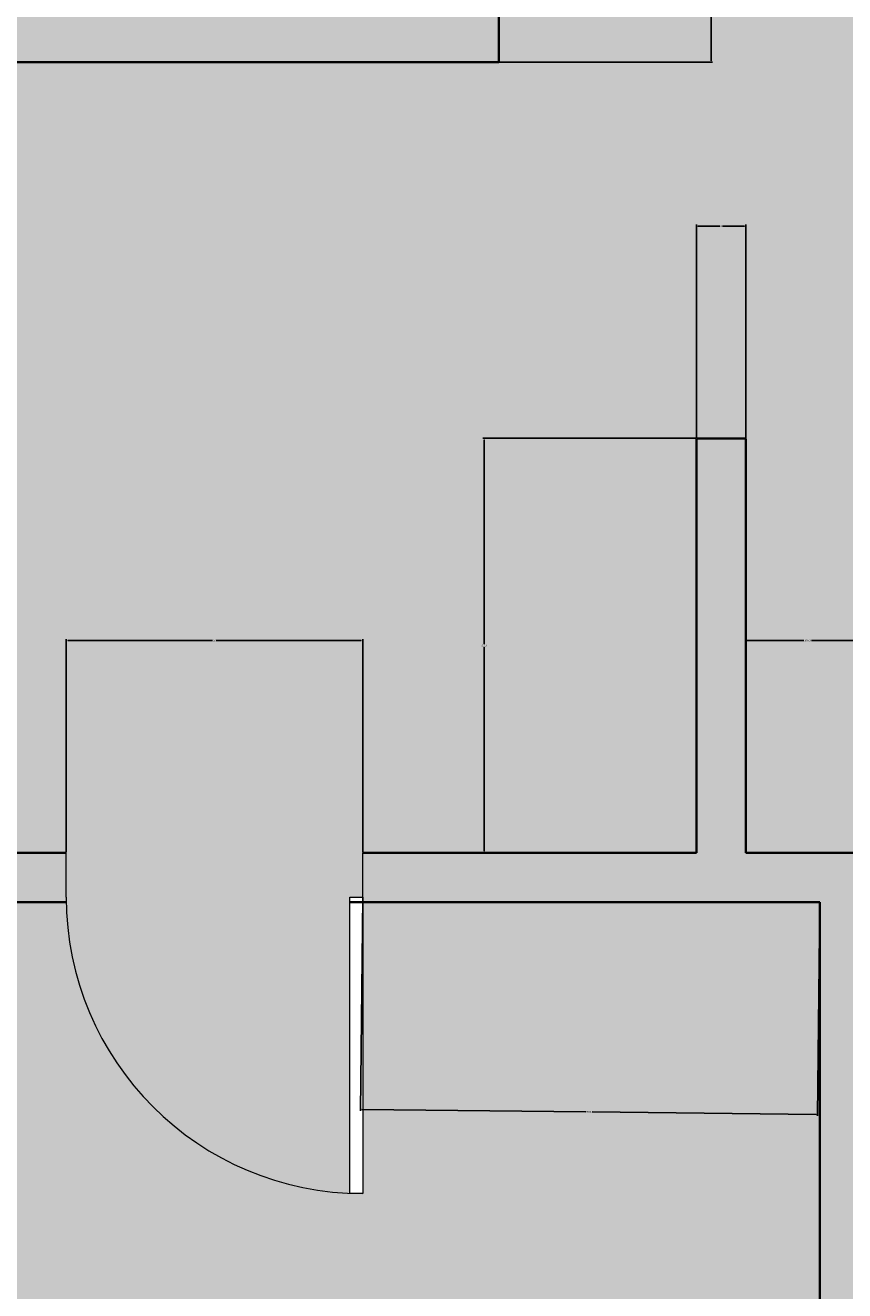
# Model space of a CAD drawing. Units: inches. Extents: x 3024 to 3952, y 1308 to 1863.
# Tile 3 of 29: x 3175 to 3275, y 1479 to 1633. Entities that reach past the tile are written whole.
import ezdxf

# ---------------------------------------------------------------- set-up
doc = ezdxf.new("R2010")
doc.units = ezdxf.units.IN
for name, color, linetype, lineweight in [('A-ANNO-DIMS', 2, 'Continuous', 18), ('A-DOOR', 4, 'Continuous', 18), ('A-FLOR-TILE-PATT', 7, 'Continuous', 13), ('A-WALL', 7, 'Continuous', 35)]:
    doc.layers.add(name, color=color, linetype=linetype, lineweight=lineweight)
doc.layers.add('A-FLOR-PATT', color=254, linetype='Continuous', lineweight=13, true_color=0xfeeab9)
doc.layers.add('A-WALL-PATT', color=254, linetype='Continuous', lineweight=13, true_color=0xcecce6)
doc.styles.get("Standard").update_dxf_attribs({"font": 'arial.ttf'})
doc.dimstyles.get("Standard").update_dxf_attribs({"dimtxt": 0.18, "dimasz": 0.18, "dimexe": 0.18, "dimexo": 0.0625, "dimgap": 0.09, "dimtad": 0, "dimtih": 1, "dimtoh": 1, "dimdec": 4, "dimzin": 0, "dimdsep": 46, "dimtxsty": 'Standard', "dimcen": 0.09, "dimadec": 0, "dimazin": 0, "dimtfac": 1, "dimtdec": 4, "dimtofl": 0, "dimtmove": 0, "dimatfit": 3, "dimfxl": 1, "dimtolj": 1, "dimtzin": 0, "dimarcsym": 0})

# ---------------------------------------------------------------- blocks, each defined once
blk = doc.blocks.new('*U2')
for p, q in [((0, 0), (0, -6)), ((40, 0), (40, -6))]:
    blk.add_line(p, q)
blk.add_lwpolyline([(0, 0), (0, 40), (1.75, 40), (1.75, 0)], close=True)
blk.add_arc((0, 0), 40, 0, 90)
blk = doc.blocks.new('*D52')
at = {"layer": 'A-ANNO-DIMS', "color": 0, "lineweight": -2, "transparency": 16777216}
for p, q in [((3180.24, 1532.67), (3180.24, 1558.56)), ((3216.24, 1532.67), (3216.24, 1558.56)), ((3180.42, 1558.38), (3198.02, 1558.38)), ((3216.06, 1558.38), (3198.46, 1558.38))]:
    blk.add_line(p, q, dxfattribs=at)
at = {"layer": 'A-ANNO-DIMS', "color": 0, "transparency": 16777216}
for points in [[(3180.42, 1558.41), (3180.42, 1558.35), (3180.24, 1558.38)], [(3216.06, 1558.41), (3216.06, 1558.35), (3216.24, 1558.38)]]:
    blk.add_solid(points, dxfattribs=at)
at = {"layer": 'Defpoints', "color": 0, "transparency": 16777216}
for p in [(3216.24, 1558.38), (3180.24, 1532.61), (3216.24, 1532.61)]:
    blk.add_point(p, dxfattribs=at)
at = {"layer": 'A-ANNO-DIMS', "color": 0, "transparency": 16777216, "insert": (3198.24, 1558.38), "char_height": 0.18, "attachment_point": 5}
blk.add_mtext('\\A1;36', dxfattribs=at)
blk = doc.blocks.new('*D55')
at = {"layer": 'A-ANNO-DIMS', "color": 0, "lineweight": -2, "transparency": 16777216}
for p, q in [((3216.24, 1527.14), (3215.96, 1501.25)), ((3271.76, 1526.54), (3271.48, 1500.65)), ((3216.14, 1501.43), (3243.33, 1501.14)), ((3271.31, 1500.83), (3244.12, 1501.13))]:
    blk.add_line(p, q, dxfattribs=at)
at = {"layer": 'A-ANNO-DIMS', "color": 0, "transparency": 16777216}
for points in [[(3216.14, 1501.46), (3216.14, 1501.4), (3215.96, 1501.43)], [(3271.31, 1500.86), (3271.31, 1500.8), (3271.49, 1500.83)]]:
    blk.add_solid(points, dxfattribs=at)
at = {"layer": 'Defpoints', "color": 0, "transparency": 16777216}
for p in [(3216.24, 1527.21), (3271.76, 1526.61), (3215.96, 1501.43)]:
    blk.add_point(p, dxfattribs=at)
at = {"layer": 'A-ANNO-DIMS', "color": 0, "transparency": 16777216, "insert": (3243.72, 1501.13), "char_height": 0.18, "attachment_point": 5}
blk.add_mtext('\\A1;55.53', dxfattribs=at)
blk = doc.blocks.new('*D59')
at = {"layer": 'A-ANNO-DIMS', "color": 0, "lineweight": -2, "transparency": 16777216}
for p, q in [((3232.83, 1649.9), (3258.72, 1649.9)), ((3258.54, 1649.72), (3258.54, 1639.43)), ((3258.54, 1628.79), (3258.54, 1639.07)), ((3232.83, 1628.61), (3258.72, 1628.61))]:
    blk.add_line(p, q, dxfattribs=at)
at = {"layer": 'A-ANNO-DIMS', "color": 0, "transparency": 16777216}
for points in [[(3258.51, 1649.72), (3258.57, 1649.72), (3258.54, 1649.9)], [(3258.51, 1628.79), (3258.57, 1628.79), (3258.54, 1628.61)]]:
    blk.add_solid(points, dxfattribs=at)
at = {"layer": 'Defpoints', "color": 0, "transparency": 16777216}
for p in [(3232.76, 1649.9), (3232.76, 1628.61), (3258.54, 1628.61)]:
    blk.add_point(p, dxfattribs=at)
at = {"layer": 'A-ANNO-DIMS', "color": 0, "transparency": 16777216, "insert": (3258.54, 1639.25), "char_height": 0.18, "attachment_point": 5}
blk.add_mtext('\\A1;21.29', dxfattribs=at)
blk = doc.blocks.new('*D64')
at = {"layer": 'A-ANNO-DIMS', "color": 0, "lineweight": -2, "transparency": 16777216}
for p, q in [((3256.7, 1582.94), (3230.81, 1582.94)), ((3230.99, 1582.76), (3230.99, 1557.95)), ((3230.99, 1532.79), (3230.99, 1557.59)), ((3256.7, 1532.61), (3230.81, 1532.61))]:
    blk.add_line(p, q, dxfattribs=at)
at = {"layer": 'A-ANNO-DIMS', "color": 0, "transparency": 16777216}
for points in [[(3230.96, 1582.76), (3231.02, 1582.76), (3230.99, 1582.94)], [(3230.96, 1532.79), (3231.02, 1532.79), (3230.99, 1532.61)]]:
    blk.add_solid(points, dxfattribs=at)
at = {"layer": 'Defpoints', "color": 0, "transparency": 16777216}
for p in [(3230.99, 1582.94), (3256.76, 1582.94), (3256.76, 1532.61)]:
    blk.add_point(p, dxfattribs=at)
at = {"layer": 'A-ANNO-DIMS', "color": 0, "transparency": 16777216, "insert": (3230.99, 1557.77), "char_height": 0.18, "attachment_point": 5}
blk.add_mtext('\\A1;50.33', dxfattribs=at)
blk = doc.blocks.new('*D65')
at = {"layer": 'A-ANNO-DIMS', "color": 0, "lineweight": -2, "transparency": 16777216}
for p, q in [((3262.76, 1532.67), (3262.76, 1558.56)), ((3277.76, 1532.67), (3277.76, 1558.56)), ((3262.94, 1558.38), (3269.81, 1558.38)), ((3277.58, 1558.38), (3270.72, 1558.38))]:
    blk.add_line(p, q, dxfattribs=at)
at = {"layer": 'A-ANNO-DIMS', "color": 0, "transparency": 16777216}
for points in [[(3262.94, 1558.41), (3262.94, 1558.35), (3262.76, 1558.38)], [(3277.58, 1558.41), (3277.58, 1558.35), (3277.76, 1558.38)]]:
    blk.add_solid(points, dxfattribs=at)
at = {"layer": 'Defpoints', "color": 0, "transparency": 16777216}
for p in [(3277.76, 1558.38), (3262.76, 1532.61), (3277.76, 1532.61)]:
    blk.add_point(p, dxfattribs=at)
at = {"layer": 'A-ANNO-DIMS', "color": 0, "transparency": 16777216, "insert": (3270.26, 1558.38), "char_height": 0.18, "attachment_point": 5}
blk.add_mtext('\\A1;15.003', dxfattribs=at)
blk = doc.blocks.new('*D66')
at = {"layer": 'A-ANNO-DIMS', "color": 0, "lineweight": -2, "transparency": 16777216}
for p, q in [((3256.76, 1583), (3256.76, 1608.89)), ((3256.94, 1608.71), (3259.61, 1608.71)), ((3262.58, 1608.71), (3259.91, 1608.71)), ((3262.76, 1583), (3262.76, 1608.89))]:
    blk.add_line(p, q, dxfattribs=at)
at = {"layer": 'A-ANNO-DIMS', "color": 0, "transparency": 16777216}
for points in [[(3256.94, 1608.74), (3256.94, 1608.68), (3256.76, 1608.71)], [(3262.58, 1608.74), (3262.58, 1608.68), (3262.76, 1608.71)]]:
    blk.add_solid(points, dxfattribs=at)
at = {"layer": 'Defpoints', "color": 0, "transparency": 16777216}
for p in [(3262.76, 1608.71), (3256.76, 1582.94), (3262.76, 1582.94)]:
    blk.add_point(p, dxfattribs=at)
at = {"layer": 'A-ANNO-DIMS', "color": 0, "transparency": 16777216, "insert": (3259.76, 1608.71), "char_height": 0.18, "attachment_point": 5}
blk.add_mtext('\\A1;6', dxfattribs=at)

msp = doc.modelspace()

# ---------------------------------------------------------------- hatches: boundary and pattern name
at = {"layer": 'A-FLOR-PATT', "transparency": 33554528}
h = msp.add_hatch(color=256, dxfattribs=at)
h.dxf.hatch_style = 1
h.paths.add_polyline_path([(3460.764, 1688.6064), (3412.764, 1688.6064), (3412.764, 1694.6064), (3460.764, 1694.6064), (3460.764, 1778.6064), (3406.764, 1778.6064), (3406.764, 1759.9514), (3318.2981, 1759.9514), (3318.2981, 1658.6064), (3322.5356, 1658.6064), (3322.5356, 1652.6064), (3292.764, 1652.6064), (3292.764, 1778.6064), (3106.764, 1778.6064), (3106.764, 1628.6064), (3172.764, 1628.6064), (3172.764, 1532.6064), (3166.764, 1532.6064), (3166.764, 1628.6064), (3106.764, 1628.6064), (3106.764, 1356.8452), (3202.812, 1356.8452), (3202.812, 1354.2534), (3202.812, 1353.8388), (3202.812, 1351.1212), (3202.812, 1347.8452), (3277.764, 1347.8452), (3277.764, 1353.8452), (3277.764, 1356.8452), (3277.764, 1442.6064), (3460.764, 1442.6064)])
h.paths.add_polyline_path([(3216.238, 1527.2064), (3216.238, 1491.2064), (3214.663, 1491.2064), (3214.663, 1491.2409, -0.39662236), (3180.243, 1526.6064), (3163.0285, 1526.6064), (3163.0285, 1531.1064), (3161.716, 1531.1064), (3161.716, 1561.1064), (3163.0285, 1561.1064), (3163.0285, 1531.1064), (3163.0285, 1526.6064), (3180.243, 1526.6064, 0.39662236), (3214.663, 1491.2409), (3214.663, 1527.2064)], flags=16)
h.paths.add_polyline_path([(3227.364, 1649.8972), (3191.364, 1649.8972), (3191.364, 1651.4722), (3227.364, 1651.4722)], flags=16)
h.paths.add_polyline_path([(3323.1172, 1606.7362), (3323.8545, 1606.8514), (3323.8545, 1594.8241), (3323.1172, 1594.9393)], flags=16)
h.paths.add_polyline_path([(3324.2232, 1606.909), (3330.1216, 1607.8307), (3330.1216, 1614.1093), (3339.3495, 1614.1093), (3340.2711, 1620.0078), (3352.4136, 1620.0078), (3353.3353, 1614.1093), (3359.9941, 1614.1093), (3360.9157, 1620.0078), (3373.0582, 1620.0078), (3373.9799, 1614.1093), (3383.2077, 1614.1093), (3383.2077, 1607.8307), (3389.1062, 1606.909), (3389.1062, 1594.7665), (3383.2077, 1593.8449), (3383.2077, 1587.5663), (3373.9799, 1587.5663), (3373.0583, 1581.6678), (3360.9157, 1581.6678), (3359.9941, 1587.5663), (3353.3353, 1587.5663), (3352.4136, 1581.6678), (3340.2711, 1581.6678), (3339.3495, 1587.5663), (3330.1216, 1587.5663), (3330.1216, 1593.8449), (3324.2232, 1594.7665)], flags=16)
h.paths.add_polyline_path([(3236.1584, 1693.1064), (3236.1584, 1723.1064), (3237.4709, 1723.1064), (3237.4709, 1693.1064)], flags=16)
h.paths.add_polyline_path([(3373.2158, 1600.6847), (3373.7965, 1600.7303), (3374.3268, 1600.7874), (3374.8132, 1600.8531), (3375.2621, 1600.9247), (3375.6801, 1600.9991), (3376.0736, 1601.0735), (3376.6855, 1601.19), (3377.366, 1601.3023), (3378.0667, 1601.3814), (3378.8026, 1601.4123), (3379.5865, 1601.3839), (3380.4537, 1601.2948), (3381.301, 1601.1717), (3382.0317, 1601.0433), (3382.4398, 1600.9607), (3382.6252, 1600.9201), (3382.919, 1600.8507), (3382.9044, 1600.8531), (3382.842, 1600.8678), (3382.7541, 1600.8896), (3382.6252, 1600.9201), (3382.4398, 1600.9607), (3382.1868, 1601.0119), (3381.8738, 1601.0711), (3381.5125, 1601.1346), (3381.1149, 1601.1988), (3380.6928, 1601.2601), (3380.2581, 1601.3149), (3379.8226, 1601.3597), (3379.3984, 1601.3908), (3378.9944, 1601.4054), (3378.6092, 1601.4042), (3378.2384, 1601.3886), (3377.8777, 1601.36), (3377.5227, 1601.32), (3377.1691, 1601.2698), (3376.8127, 1601.211), (3376.4491, 1601.145), (3376.0736, 1601.0735), (3375.4177, 1600.9494), (3374.5542, 1600.8119), (3373.5044, 1600.6988)], flags=0)
h.paths.add_polyline_path([(3380.0253, 1596.7351), (3380.499, 1596.6659), (3380.9706, 1596.6119), (3381.4375, 1596.5791), (3381.8971, 1596.5736), (3382.5886, 1596.6167), (3382.7848, 1596.6692), (3382.1465, 1596.5706), (3381.236, 1596.5815), (3380.3199, 1596.6865)], flags=0)
h.paths.add_polyline_path([(3369.6414, 1603.9617), (3370.1589, 1604.0021), (3370.6218, 1604.0539), (3371.0335, 1604.1173), (3371.3978, 1604.1921), (3371.7181, 1604.2785), (3371.9984, 1604.3761), (3372.2441, 1604.483), (3372.4611, 1604.5972), (3372.655, 1604.7163), (3372.8317, 1604.8384), (3372.9968, 1604.9611), (3373.3703, 1605.2455), (3373.8426, 1605.5328), (3374.4624, 1605.7539), (3375.1058, 1605.8302), (3375.7221, 1605.8261), (3376.4109, 1605.76), (3377.1534, 1605.6376), (3377.8945, 1605.473), (3378.1382, 1605.409), (3377.7394, 1605.5074), (3377.3509, 1605.5937), (3376.9704, 1605.6677), (3376.5999, 1605.7288), (3376.2417, 1605.7762), (3375.8979, 1605.8092), (3375.5707, 1605.8271), (3375.2621, 1605.8291), (3374.9745, 1605.8146), (3374.7092, 1605.7832), (3374.4647, 1605.7359), (3374.239, 1605.6742), (3374.0298, 1605.5996), (3373.835, 1605.5134), (3373.6525, 1605.4171), (3373.4801, 1605.3123), (3373.3156, 1605.2002), (3373.1562, 1605.0825), (3372.7603, 1604.781), (3372.236, 1604.4588), (3371.5738, 1604.2283), (3370.8493, 1604.0794), (3369.9262, 1603.976)], flags=0)
h.paths.add_polyline_path([(3366.7533, 1606.5832), (3367.1713, 1606.5519), (3367.5378, 1606.5374), (3367.8568, 1606.5394), (3368.1325, 1606.5573), (3368.3694, 1606.5903), (3368.5717, 1606.6377), (3368.7438, 1606.6988), (3368.89, 1606.7728), (3369.0146, 1606.8591), (3369.121, 1606.9568), (3369.2094, 1607.0646), (3369.2792, 1607.181), (3369.3295, 1607.3046), (3369.3596, 1607.4339), (3369.3688, 1607.5676), (3369.3565, 1607.7042), (3369.3218, 1607.8422), (3369.2649, 1607.9804), (3369.1893, 1608.1187), (3369.0993, 1608.2569), (3368.9992, 1608.3952), (3368.8934, 1608.5334), (3368.7861, 1608.6717), (3368.6817, 1608.8099), (3368.4212, 1609.1804), (3368.2685, 1609.7106), (3368.4883, 1610.1814), (3369.0537, 1610.4604), (3369.6717, 1610.5097), (3370.2812, 1610.3612), (3370.4805, 1610.2968), (3370.1882, 1610.3839), (3369.9284, 1610.4472), (3369.6905, 1610.4842), (3369.4662, 1610.4933), (3369.2555, 1610.4765), (3369.0608, 1610.4367), (3368.884, 1610.3767), (3368.7274, 1610.2994), (3368.5931, 1610.2077), (3368.4833, 1610.1045), (3368.4002, 1609.9927), (3368.3451, 1609.8747), (3368.3166, 1609.7517), (3368.3127, 1609.6244), (3368.331, 1609.4935), (3368.3696, 1609.3597), (3368.4261, 1609.2237), (3368.4985, 1609.0863), (3368.5845, 1608.9482), (3368.6817, 1608.8099), (3368.7861, 1608.6717), (3368.8934, 1608.5334), (3368.9992, 1608.3952), (3369.0993, 1608.2569), (3369.3398, 1607.8876), (3369.3941, 1607.2896), (3368.9774, 1606.7817), (3368.3928, 1606.5742), (3367.7162, 1606.5303), (3367.0044, 1606.5585)], flags=0)
h.paths.add_polyline_path([(3362.1859, 1610.2589), (3362.5478, 1610.2845), (3362.8348, 1610.3275), (3363.0585, 1610.3863), (3363.2303, 1610.4595), (3363.3619, 1610.5457), (3363.463, 1610.6432), (3363.5376, 1610.7502), (3363.5876, 1610.8643), (3363.6153, 1610.9834), (3363.6229, 1611.1055), (3363.6125, 1611.2283), (3363.5861, 1611.3496), (3363.5462, 1611.4673), (3363.4949, 1611.5797), (3363.4358, 1611.6871), (3363.3723, 1611.7902), (3363.3081, 1611.8897), (3363.2468, 1611.9863), (3363.192, 1612.0808), (3363.0258, 1612.4261), (3363.3371, 1612.8672), (3363.9008, 1612.9782), (3364.4822, 1612.9641), (3365.1098, 1612.9074), (3365.328, 1612.8805), (3364.9615, 1612.9208), (3364.6426, 1612.9496), (3364.3668, 1612.9669), (3364.1299, 1612.9726), (3363.9276, 1612.9669), (3363.7555, 1612.9496), (3363.6093, 1612.9208), (3363.4848, 1612.8805), (3363.3782, 1612.8289), (3363.2889, 1612.7672), (3363.2169, 1612.6969), (3363.1622, 1612.6193), (3363.1247, 1612.5361), (3363.1046, 1612.4484), (3363.1017, 1612.358), (3363.1161, 1612.266), (3363.1472, 1612.1738), (3363.192, 1612.0808), (3363.2468, 1611.9863), (3363.3081, 1611.8897), (3363.3723, 1611.7902), (3363.4358, 1611.6871), (3363.6363, 1611.323), (3363.5979, 1610.7003), (3363.0863, 1610.3651), (3362.3983, 1610.2622)], flags=0)
h.paths.add_polyline_path([(3352.356, 1581.2991), (3352.2408, 1580.5618), (3340.4439, 1580.5618), (3340.3287, 1581.2991)], flags=16)
h.paths.add_polyline_path([(3340.4439, 1621.1137), (3352.2408, 1621.1137), (3352.356, 1620.3764), (3340.3287, 1620.3764)], flags=16)
h.paths.add_polyline_path([(3278.4282, 1504.7424), (3290.3831, 1504.7424), (3290.3831, 1502.7499), (3291.0473, 1502.7499), (3291.0473, 1494.7799), (3290.3831, 1494.7799), (3290.3831, 1494.1158), (3291.0473, 1494.1158), (3291.0473, 1486.1458), (3290.3831, 1486.1458), (3290.3831, 1484.1533), (3291.0473, 1484.1533), (3291.0473, 1483.4892, -0.09090909), (3291.0473, 1468.8776), (3291.0473, 1468.2135), (3290.3831, 1468.2135), (3290.3831, 1464.8926), (3278.4282, 1464.8926), (3278.4282, 1472.8626), (3277.764, 1473.5268), (3277.764, 1478.84), (3278.4282, 1479.5042)], flags=16)
h.paths.add_polyline_path([(3278.7603, 1504.4103), (3290.051, 1504.4103), (3290.051, 1465.2247), (3278.7603, 1465.2247)], flags=0)
h.paths.add_polyline_path([(3123.904, 1600.7821), (3117.9039, 1602.7821), (3117.9039, 1599.7821), (3119.4039, 1599.7821), (3119.4039, 1596.7821), (3118.4039, 1596.7821), (3118.4039, 1598.7821), (3117.9039, 1598.7821), (3117.9039, 1596.2821), (3109.9039, 1596.2821), (3109.9039, 1617.2821), (3117.9039, 1617.2821), (3117.9039, 1610.7821), (3123.9038, 1612.7821, -0.70257121), (3137.9039, 1606.7822, -0.70256205)], flags=16)
h.paths.add_polyline_path([(3123.9039, 1602.7822), (3123.9039, 1610.7822, -0.73453329), (3136.9039, 1606.7822, -0.73452973)], flags=0)
h.paths.add_polyline_path([(3177.972, 1689.6473), (3109.2405, 1689.6473), (3109.2405, 1741.1959), (3177.972, 1741.1959)], flags=16)
h.paths.add_polyline_path([(3373.0006, 1581.2991), (3372.8854, 1580.5618), (3361.0885, 1580.5618), (3360.9733, 1581.2991)], flags=16)
h.paths.add_polyline_path([(3361.0885, 1621.1137), (3372.8854, 1621.1137), (3373.0006, 1620.3764), (3360.9733, 1620.3764)], flags=16)
h.paths.add_polyline_path([(3116.9039, 1598.2821, -0.41421356), (3116.1539, 1597.2821), (3111.9039, 1597.2821, -0.41421356), (3110.9039, 1598.0321), (3110.9039, 1615.2821, -0.41421356), (3111.6539, 1616.2821), (3115.9039, 1616.2821, -0.41421356), (3116.9039, 1615.5321)], flags=0)
h.paths.add_polyline_path([(3121.6122, 1728.1369), (3121.6122, 1696.5205), (3110.2715, 1696.5205), (3110.2715, 1714.3906), (3121.6122, 1714.3906), (3121.6122, 1716.4526), (3110.2715, 1716.4526), (3110.2715, 1734.3228), (3123.3304, 1734.3228), (3123.3304, 1729.8552), (3134.6711, 1741.1959), (3134.6711, 1728.1369)], flags=0)
h.paths.add_polyline_path([(3389.4748, 1606.8514), (3390.2122, 1606.7362), (3390.2122, 1594.9393), (3389.4748, 1594.8241)], flags=16)
h.paths.add_polyline_path([(3257.6842, 1762.8281), (3259.6842, 1768.8281), (3256.6842, 1768.8281), (3256.6842, 1767.3281), (3253.6842, 1767.3281), (3253.6842, 1768.3281), (3255.6842, 1768.3281), (3255.6842, 1768.8281), (3253.1842, 1768.8281), (3253.1842, 1776.8281), (3274.1842, 1776.8281), (3274.1842, 1768.8281), (3267.6842, 1768.8281), (3269.6842, 1762.8282, -0.70257121), (3263.6843, 1748.8282, -0.70256205)], flags=16)
h.paths.add_polyline_path([(3259.6842, 1762.8281), (3267.6843, 1762.8281, -0.73453329), (3263.6842, 1749.8282, -0.73452973)], flags=0)
h.paths.add_polyline_path([(3411.264, 1715.6064), (3411.264, 1716.9189), (3441.264, 1716.9189), (3441.264, 1715.6064)], flags=16)
h.paths.add_polyline_path([(3178.3806, 1449.1876), (3178.3806, 1397.639), (3109.6491, 1397.639), (3109.6491, 1449.1876)], flags=16)
h.paths.add_polyline_path([(3397.1501, 1541.7146), (3419.6183, 1541.7146), (3419.6183, 1496.7783), (3397.1501, 1496.7783)], flags=16)
h.paths.add_polyline_path([(3254.1842, 1770.5781), (3254.1842, 1774.8281, -0.41421356), (3254.9342, 1775.8281), (3272.1842, 1775.8281, -0.41421356), (3273.1842, 1775.0781), (3273.1842, 1770.8281, -0.41421356), (3272.4342, 1769.8281), (3255.1842, 1769.8281, -0.41421356)], flags=0)
h.paths.add_polyline_path([(3403.672, 1500.7601), (3403.6016, 1500.3997), (3403.5328, 1500.0441), (3403.4662, 1499.6867), (3403.4027, 1499.3226), (3403.3464, 1498.9532), (3403.3025, 1498.5811), (3403.2759, 1498.2091), (3403.2714, 1497.8401), (3403.3064, 1497.2813), (3403.3491, 1497.1219), (3403.2689, 1497.6395), (3403.2778, 1498.3719), (3403.3635, 1499.0984), (3403.4889, 1499.8168), (3403.6016, 1500.3997), (3403.672, 1500.7601), (3403.744, 1501.1315), (3403.817, 1501.5205), (3403.891, 1501.9336), (3403.9656, 1502.3769), (3404.0404, 1502.8572), (3404.115, 1503.3786), (3404.2264, 1504.2311), (3404.2571, 1504.5223), (3404.1552, 1503.6598), (3404.0063, 1502.6193), (3403.8604, 1501.7518), (3403.744, 1501.1315)], flags=0)
h.paths.add_polyline_path([(3406.5868, 1505.0416), (3406.6121, 1504.5236), (3406.6492, 1504.0526), (3406.6956, 1503.624), (3406.7491, 1503.2333), (3406.8072, 1502.8759), (3406.8676, 1502.5473), (3406.9281, 1502.243), (3407.0268, 1501.7597), (3407.1416, 1501.1368), (3407.2087, 1500.3904), (3407.1804, 1499.6703), (3407.1078, 1498.9956), (3407.0074, 1498.3199), (3406.8809, 1497.6059), (3406.7403, 1496.9627), (3406.7418, 1496.9824), (3406.7491, 1497.0249), (3406.8229, 1497.3409), (3406.8364, 1497.4025), (3406.878, 1497.6078), (3406.9261, 1497.8614), (3406.9777, 1498.1526), (3407.0298, 1498.4712), (3407.0797, 1498.8068), (3407.1243, 1499.149), (3407.1607, 1499.4874), (3407.1859, 1499.8115), (3407.1978, 1500.1137), (3407.1969, 1500.3962), (3407.1841, 1500.6642), (3407.1609, 1500.9225), (3407.1284, 1501.1761), (3407.0876, 1501.43), (3407.0398, 1501.6891), (3406.9862, 1501.9585), (3406.8832, 1502.4628), (3406.7712, 1503.0713), (3406.6657, 1503.8424), (3406.5924, 1504.7735)], flags=0)
h.paths.add_polyline_path([(3409.2517, 1507.8962), (3409.2752, 1507.4282), (3409.3079, 1507.0076), (3409.3501, 1506.6314), (3409.4015, 1506.2969), (3409.4624, 1506.0009), (3409.5326, 1505.7406), (3409.6119, 1505.5128), (3409.6988, 1505.3131), (3409.7915, 1505.1368), (3409.8883, 1504.9792), (3409.9875, 1504.8356), (3410.0872, 1504.7015), (3410.1859, 1504.572), (3410.4508, 1504.2132), (3410.7205, 1503.6035), (3410.8059, 1502.8824), (3410.7619, 1502.0875), (3410.6122, 1501.2299), (3410.4402, 1500.6169), (3410.2538, 1500.0031), (3410.0536, 1499.3219), (3409.9909, 1499.0812), (3410.1761, 1499.7472), (3410.3596, 1500.3513), (3410.4512, 1500.6561), (3410.5312, 1500.9412), (3410.6013, 1501.226), (3410.6614, 1501.512), (3410.7111, 1501.7964), (3410.7496, 1502.0763), (3410.7764, 1502.3489), (3410.7909, 1502.6114), (3410.7926, 1502.8608), (3410.7808, 1503.0944), (3410.7553, 1503.31), (3410.7169, 1503.5087), (3410.6667, 1503.6921), (3410.6061, 1503.8621), (3410.5361, 1504.0203), (3410.4578, 1504.1686), (3410.3726, 1504.3088), (3410.2815, 1504.4424), (3410.1859, 1504.572), (3410.0872, 1504.7015), (3409.859, 1505.0083), (3409.5943, 1505.5117), (3409.4266, 1506.1336), (3409.324, 1506.8011), (3409.2586, 1507.6407)], flags=0)
h.paths.add_polyline_path([(3411.4914, 1510.5878), (3411.4432, 1510.1586), (3411.4054, 1509.775), (3411.38, 1509.4354), (3411.3681, 1509.1376), (3411.3698, 1508.8784), (3411.3843, 1508.6542), (3411.4112, 1508.4618), (3411.4497, 1508.2974), (3411.4994, 1508.1575), (3411.5595, 1508.0388), (3411.6296, 1507.9375), (3411.7097, 1507.851), (3411.802, 1507.7792), (3411.9096, 1507.7225), (3412.0353, 1507.6817), (3412.1821, 1507.6572), (3412.3528, 1507.6496), (3412.5505, 1507.6597), (3412.778, 1507.6879), (3413.0364, 1507.7341), (3413.3194, 1507.7955), (3413.6188, 1507.8687), (3413.9264, 1507.95), (3414.234, 1508.036), (3414.5333, 1508.1232), (3414.8163, 1508.208), (3415.0747, 1508.287), (3415.3023, 1508.3569), (3415.5007, 1508.4158), (3415.6733, 1508.4617), (3416.1158, 1508.5538), (3416.512, 1508.2591), (3416.716, 1507.6581), (3416.61, 1507.0003), (3416.3052, 1506.3411), (3415.8928, 1505.618), (3415.7339, 1505.3633), (3415.9914, 1505.791), (3416.201, 1506.1583), (3416.3666, 1506.4739), (3416.4925, 1506.7462), (3416.5828, 1506.9838), (3416.6413, 1507.1949), (3416.6725, 1507.3883), (3416.6799, 1507.5705), (3416.6662, 1507.7417), (3416.6339, 1507.9), (3416.5851, 1508.0436), (3416.5223, 1508.1709), (3416.4478, 1508.28), (3416.3639, 1508.3692), (3416.273, 1508.4368), (3416.1765, 1508.4815), (3416.0718, 1508.5047), (3415.9553, 1508.5079), (3415.8237, 1508.493), (3415.6733, 1508.4617), (3415.5007, 1508.4158), (3415.3327, 1508.3659), (3414.6495, 1508.157), (3414.0606, 1507.9855), (3413.4456, 1507.8229), (3412.8838, 1507.701), (3412.5505, 1507.6597), (3412.0748, 1507.6354), (3411.595, 1507.8883), (3411.398, 1508.4429), (3411.3624, 1508.9927), (3411.3854, 1509.5711), (3411.4578, 1510.3071)], flags=0)
h.paths.add_polyline_path([(3135.0797, 1449.1876), (3135.0797, 1436.1286), (3122.0208, 1436.1286), (3122.0208, 1404.5122), (3110.6801, 1404.5122), (3110.6801, 1422.3823), (3122.0208, 1422.3823), (3122.0208, 1424.4443), (3110.6801, 1424.4443), (3110.6801, 1442.3145), (3123.739, 1442.3145), (3123.739, 1437.8469)], flags=0)
h.paths.add_polyline_path([(3416.4944, 1514.2949), (3416.4837, 1513.8511), (3416.4893, 1513.4867), (3416.5102, 1513.1926), (3416.5451, 1512.9593), (3416.5929, 1512.7775), (3416.6524, 1512.6379), (3416.7224, 1512.531), (3416.8017, 1512.4488), (3416.8886, 1512.3882), (3416.9813, 1512.3476), (3417.0781, 1512.3251), (3417.1773, 1512.3189), (3417.277, 1512.3274), (3417.3757, 1512.3488), (3417.4713, 1512.3813), (3417.5627, 1512.4229), (3417.65, 1512.471), (3417.7338, 1512.5225), (3417.8146, 1512.5747), (3417.8931, 1512.6245), (3417.9699, 1512.6691), (3418.2968, 1512.8265), (3418.6505, 1512.4645), (3418.7037, 1511.9342), (3418.6693, 1511.3839), (3418.6076, 1510.8228), (3418.5777, 1510.5927), (3418.6197, 1510.9333), (3418.6525, 1511.2311), (3418.6759, 1511.4903), (3418.6899, 1511.7144), (3418.6946, 1511.9069), (3418.6899, 1512.0713), (3418.6759, 1512.2112), (3418.6525, 1512.33), (3418.6197, 1512.4311), (3418.5778, 1512.5177), (3418.5276, 1512.5903), (3418.4705, 1512.6488), (3418.4075, 1512.6933), (3418.3399, 1512.7237), (3418.2686, 1512.7401), (3418.1951, 1512.7424), (3418.1204, 1512.7307), (3418.0455, 1512.7055), (3417.9792, 1512.6736), (3417.65, 1512.471), (3417.5627, 1512.4229), (3417.4713, 1512.3813), (3417.3757, 1512.3488), (3417.277, 1512.3274), (3416.878, 1512.2936), (3416.5757, 1512.7549), (3416.492, 1513.3145), (3416.4808, 1514.0384)], flags=0)
h.paths.add_polyline_path([(3392.8223, 1481.9454), (3396.7707, 1481.9454), (3396.7707, 1480.9201), (3428.3585, 1480.9201), (3428.3585, 1481.9454), (3432.3069, 1481.9454), (3432.3069, 1464.8354, -0.26666697), (3392.8223, 1464.8354)], flags=16)
h.paths.add_polyline_path([(3431.203, 1547.5428), (3450.8613, 1547.5428, -0.19047621), (3450.8614, 1484.031), (3431.203, 1484.031), (3431.203, 1488.5675), (3432.3809, 1488.5675), (3432.3809, 1543.0062), (3431.203, 1543.0062)], flags=16)
h.paths.add_polyline_path([(3451.9233, 1524.86, -0.04962821), (3451.9233, 1506.7138), (3446.7921, 1506.7138), (3446.7921, 1524.86)], flags=0)
h.paths.add_polyline_path([(3460.764, 1436.6064), (3277.764, 1436.6064), (3277.764, 1356.8452), (3277.764, 1353.8452), (3460.764, 1353.8452)], flags=17)
h.paths.add_polyline_path([(3121.3033, 1577.378), (3153.693, 1577.378), (3153.693, 1586.6752), (3121.3033, 1586.6752)], flags=24)
h.paths.add_polyline_path([(3164.1457, 1464.1276), (3210.4801, 1464.1276), (3210.4801, 1473.4247), (3164.1457, 1473.4247)], flags=24)
h.paths.add_polyline_path([(3343.1909, 1505.8863), (3373.7236, 1505.8863), (3373.7236, 1515.1773), (3343.1909, 1515.1773)], flags=24)
h.paths.add_polyline_path([(3337.6353, 1564.2926), (3370.0189, 1564.2926), (3370.0189, 1573.5836), (3337.6353, 1573.5836)], flags=24)
h.paths.add_polyline_path([(3419.204, 1753.8578), (3453.3997, 1753.8578), (3453.3997, 1762.9956), (3419.204, 1762.9956)], flags=24)
h.paths.add_polyline_path([(3341.2523, 1701.0246), (3381.0761, 1701.0246), (3381.0761, 1710.3156), (3341.2523, 1710.3156)], flags=24)
h.paths.add_polyline_path([(3245.8895, 1726.2997), (3278.2793, 1726.2997), (3278.2793, 1735.5968), (3245.8895, 1735.5968)], flags=24)
h.paths.add_polyline_path([(3128.8045, 1668.6736), (3175.1389, 1668.6736), (3175.1389, 1677.9707), (3128.8045, 1677.9707)], flags=24)
h.paths.add_polyline_path([(3345.9997, 1396.0062), (3389.09, 1396.0062), (3389.09, 1405.3033), (3345.9997, 1405.3033)], flags=24)
at = {"layer": 'A-FLOR-TILE-PATT', "transparency": 33554569}
h = msp.add_hatch(dxfattribs=at)
h.set_pattern_fill('ANGLE', color=256, scale=2)
h.set_pattern_definition([(0, (0, 0), (0, 13.97), [10.16, -3.81]), (90, (0, 0), (-13.97, 9e-16), [10.16, -3.81])])
h.paths.add_polyline_path([(3292.764, 1778.6064), (3232.764, 1778.6064), (3232.764, 1694.6064), (3236.1584, 1694.6064), (3236.1584, 1723.1064), (3237.4709, 1723.1064), (3237.4709, 1723.0777, -0.38700389), (3266.1209, 1694.6064), (3292.764, 1694.6064)])
h.paths.add_polyline_path([(3263.6843, 1748.8282, -0.70256205), (3257.6842, 1762.8281), (3259.6842, 1768.8281), (3256.6842, 1768.8281), (3256.6842, 1767.3281), (3253.6842, 1767.3281), (3253.6842, 1768.3281), (3255.6842, 1768.3281), (3255.6842, 1768.8281), (3253.1842, 1768.8281), (3253.1842, 1776.8281), (3274.1842, 1776.8281), (3274.1842, 1768.8281), (3267.6842, 1768.8281), (3269.6842, 1762.8282, -0.70257121)], flags=16)
h.paths.add_polyline_path([(3263.6842, 1749.8282, -0.73452973), (3259.6842, 1762.8281), (3267.6843, 1762.8281, -0.73453329)], flags=0)
h.paths.add_polyline_path([(3255.1842, 1769.8281, -0.41421356), (3254.1842, 1770.5781), (3254.1842, 1774.8281, -0.41421356), (3254.9342, 1775.8281), (3272.1842, 1775.8281, -0.41421356), (3273.1842, 1775.0781), (3273.1842, 1770.8281, -0.41421356), (3272.4342, 1769.8281)], flags=0)
h.paths.add_polyline_path([(3460.764, 1436.6064), (3277.764, 1436.6064), (3277.764, 1356.8452), (3277.764, 1353.8452), (3460.764, 1353.8452)])
h.paths.add_polyline_path([(3166.764, 1628.6064), (3106.764, 1628.6064), (3106.764, 1532.6064), (3133.066, 1532.6064, -0.38700389), (3161.716, 1561.0777), (3161.716, 1561.1064), (3163.0285, 1561.1064), (3163.0285, 1532.6064), (3166.764, 1532.6064)])
h.paths.add_polyline_path([(3123.904, 1600.7821), (3117.9039, 1602.7821), (3117.9039, 1599.7821), (3119.4039, 1599.7821), (3119.4039, 1596.7821), (3118.4039, 1596.7821), (3118.4039, 1598.7821), (3117.9039, 1598.7821), (3117.9039, 1596.2821), (3109.9039, 1596.2821), (3109.9039, 1617.2821), (3117.9039, 1617.2821), (3117.9039, 1610.7821), (3123.9038, 1612.7821, -0.70257121), (3137.9039, 1606.7822, -0.70256205)], flags=16)
h.paths.add_polyline_path([(3123.9039, 1602.7822), (3123.9039, 1610.7822, -0.73453329), (3136.9039, 1606.7822, -0.73452973)], flags=0)
h.paths.add_polyline_path([(3116.1539, 1597.2821), (3111.9039, 1597.2821, -0.41421356), (3110.9039, 1598.0321), (3110.9039, 1615.2821, -0.41421356), (3111.6539, 1616.2821), (3115.9039, 1616.2821, -0.41421356), (3116.9039, 1615.5321), (3116.9039, 1598.2821, -0.41421356)], flags=0)
h.paths.add_polyline_path([(3245.8895, 1726.2997), (3278.2793, 1726.2997), (3278.2793, 1735.5968), (3245.8895, 1735.5968)], flags=24)
h.paths.add_polyline_path([(3345.9997, 1396.0062), (3389.09, 1396.0062), (3389.09, 1405.3033), (3345.9997, 1405.3033)], flags=24)
h.paths.add_polyline_path([(3121.3033, 1577.378), (3153.693, 1577.378), (3153.693, 1586.6752), (3121.3033, 1586.6752)], flags=24)
at = {"layer": 'A-WALL-PATT'}
h = msp.add_hatch(color=256, dxfattribs=at)
h.dxf.hatch_style = 1
h.paths.add_polyline_path([(3106.764, 1778.6064), (3140.5977, 1778.6064), (3140.5977, 1781.8824), (3140.5977, 1784.6), (3140.5977, 1787.6064), (3097.764, 1787.6064), (3097.764, 1590.213), (3101.04, 1590.213), (3103.7576, 1590.213), (3106.764, 1590.213)])
h.paths.add_polyline_path([(3253.5314, 1781.8824), (3253.5314, 1784.6), (3253.5314, 1787.6064), (3194.6826, 1787.6064), (3194.6826, 1785.0146), (3194.6826, 1784.6), (3194.6826, 1781.8824), (3194.6826, 1778.6064), (3253.5314, 1778.6064)])
h.paths.add_polyline_path([(3333.856, 1782.2838), (3333.856, 1784.7474), (3333.856, 1787.6064), (3272.0523, 1787.6064), (3272.0523, 1785.0146), (3272.0523, 1784.6), (3272.0523, 1781.8824), (3272.0523, 1778.6064), (3333.856, 1778.6064)])
h.paths.add_polyline_path([(3428.8344, 1784.6), (3428.8344, 1787.6064), (3378.3947, 1787.6064), (3378.3947, 1784.7474), (3378.3947, 1782.2838), (3378.3947, 1778.6064), (3428.8344, 1778.6064), (3428.8344, 1781.8824)], flags=17)
h.paths.add_polyline_path([(3469.764, 1787.6064), (3451.9386, 1787.6064), (3451.9386, 1785.0146), (3451.9386, 1784.6), (3451.9386, 1781.8824), (3451.9386, 1778.6064), (3460.764, 1778.6064), (3460.764, 1353.8452), (3277.764, 1353.8452), (3277.764, 1347.8452), (3469.764, 1347.8452), (3469.764, 1353.8452)])
h.paths.add_polyline_path([(3106.764, 1571.6922), (3104.1722, 1571.6922), (3103.7576, 1571.6922), (3101.04, 1571.6922), (3097.764, 1571.6922), (3097.764, 1347.8452), (3148.7271, 1347.8452), (3148.7271, 1351.1212), (3148.7271, 1353.8388), (3148.7271, 1356.8452), (3106.764, 1356.8452)])
h.paths.add_polyline_path([(3277.764, 1532.6064), (3262.7605, 1532.6064), (3262.7605, 1582.9359), (3256.7605, 1582.9359), (3256.7605, 1532.6064), (3244.2116, 1532.6064), (3216.238, 1532.6064), (3216.238, 1527.2064), (3216.238, 1526.6064), (3271.764, 1526.6064), (3271.764, 1356.8452), (3202.812, 1356.8452), (3202.812, 1354.2534), (3202.812, 1353.8388), (3202.812, 1351.1212), (3202.812, 1347.8452), (3277.764, 1347.8452), (3277.764, 1353.8452), (3277.764, 1356.8452)])
h.paths.add_polyline_path([(3180.238, 1532.6064), (3163.0285, 1532.6064), (3163.0285, 1531.1064), (3163.0285, 1526.6064), (3180.243, 1526.6064, -0.00416688), (3180.238, 1527.2064)])
h.paths.add_polyline_path([(3133.0285, 1531.1064, -0.01250587), (3133.066, 1532.6064), (3106.764, 1532.6064), (3106.764, 1526.6064), (3133.0285, 1526.6064)], flags=17)
h.paths.add_polyline_path([(3172.764, 1628.6064), (3166.764, 1628.6064), (3166.764, 1532.6064), (3172.764, 1532.6064)])
h.paths.add_polyline_path([(3232.764, 1649.8972), (3227.364, 1649.8972), (3226.764, 1649.8972), (3226.764, 1634.6064), (3106.764, 1634.6064), (3106.764, 1628.6064), (3232.764, 1628.6064)])

# ---------------------------------------------------------------- linework, layer by layer
at = {"layer": 'A-WALL'}
for p, q in [((3232.764, 1628.6064), (3232.764, 1649.8972)), ((3106.764, 1628.6064), (3232.764, 1628.6064)), ((3262.7605, 1582.9359), (3256.7605, 1582.9359)), ((3256.7605, 1582.9359), (3256.7605, 1532.6064)), ((3262.7605, 1532.6064), (3262.7605, 1582.9359)), ((3161.716, 1532.6064), (3180.238, 1532.6064)), ((3216.238, 1532.6064), (3256.7605, 1532.6064)), ((3244.2116, 1532.6064), (3256.7605, 1532.6064)), ((3262.7605, 1532.6064), (3277.764, 1532.6064)), ((3163.0285, 1526.6064), (3180.243, 1526.6064)), ((3214.663, 1526.6064), (3271.764, 1526.6064)), ((3242.6366, 1526.6064), (3271.764, 1526.6064)), ((3271.764, 1356.8452), (3271.764, 1526.6064))]:
    msp.add_line(p, q, dxfattribs=at)

# ---------------------------------------------------------------- block references
at = {"layer": 'A-DOOR', "xscale": 0.9, "yscale": 0.9, "zscale": 0.9, "rotation": 180}
msp.add_blockref('*U2', (3216.238, 1527.2064), dxfattribs=at)

# ---------------------------------------------------------------- dimensions: what is measured, and where the dimension line sits
at = {"layer": 'A-ANNO-DIMS'}
for base, p1, p2, angle, picture, middle in [((3258.539, 1628.6064), (3232.764, 1649.8972), (3232.764, 1628.6064), 270, '*D59', (3258.539, 1639.2518)), ((3230.9855, 1582.9359), (3256.7605, 1532.6064), (3256.7605, 1582.9359), 90, '*D64', (3230.9855, 1557.7711)), ((3215.9595, 1501.4329), (3271.764, 1526.6064), (3216.238, 1527.2064), 179.3809, '*D55', (3243.7225, 1501.1329))]:
    dim = msp.add_linear_dim(base=base, p1=p1, p2=p2, angle=angle, dimstyle='Standard', override={"dimdec": 2, "dimlfac": 1, "dimrnd": 0, "dimzin": 0, "dimdsep": 46, "dimlunit": 2}, dxfattribs=at)
    dim.commit()
    dim.dimension.update_dxf_attribs({"geometry": picture, "text_midpoint": middle})
for base, p1, p2, override, picture, middle in [((3262.7605, 1608.7109), (3256.7605, 1582.9359), (3262.7605, 1582.9359), {"dimdec": 0, "dimlfac": 1, "dimrnd": 0, "dimzin": 0, "dimdsep": 46, "dimlunit": 2}, '*D66', (3259.7605, 1608.7109)), ((3216.238, 1558.3814), (3180.238, 1532.6064), (3216.238, 1532.6064), {"dimdec": 0, "dimlfac": 1, "dimrnd": 0, "dimzin": 0, "dimdsep": 46, "dimlunit": 2}, '*D52', (3198.238, 1558.3814)), ((3277.76402, 1558.38141), (3262.76054, 1532.6064), (3277.76402, 1532.6064), {"dimdec": 3, "dimlfac": 1, "dimrnd": 0, "dimzin": 0, "dimdsep": 46, "dimlunit": 2}, '*D65', (3270.26228, 1558.38141))]:
    dim = msp.add_linear_dim(base=base, p1=p1, p2=p2, dimstyle='Standard', override=override, dxfattribs=at)
    dim.commit()
    dim.dimension.update_dxf_attribs({"geometry": picture, "text_midpoint": middle})

doc.saveas('drawing.dxf')
